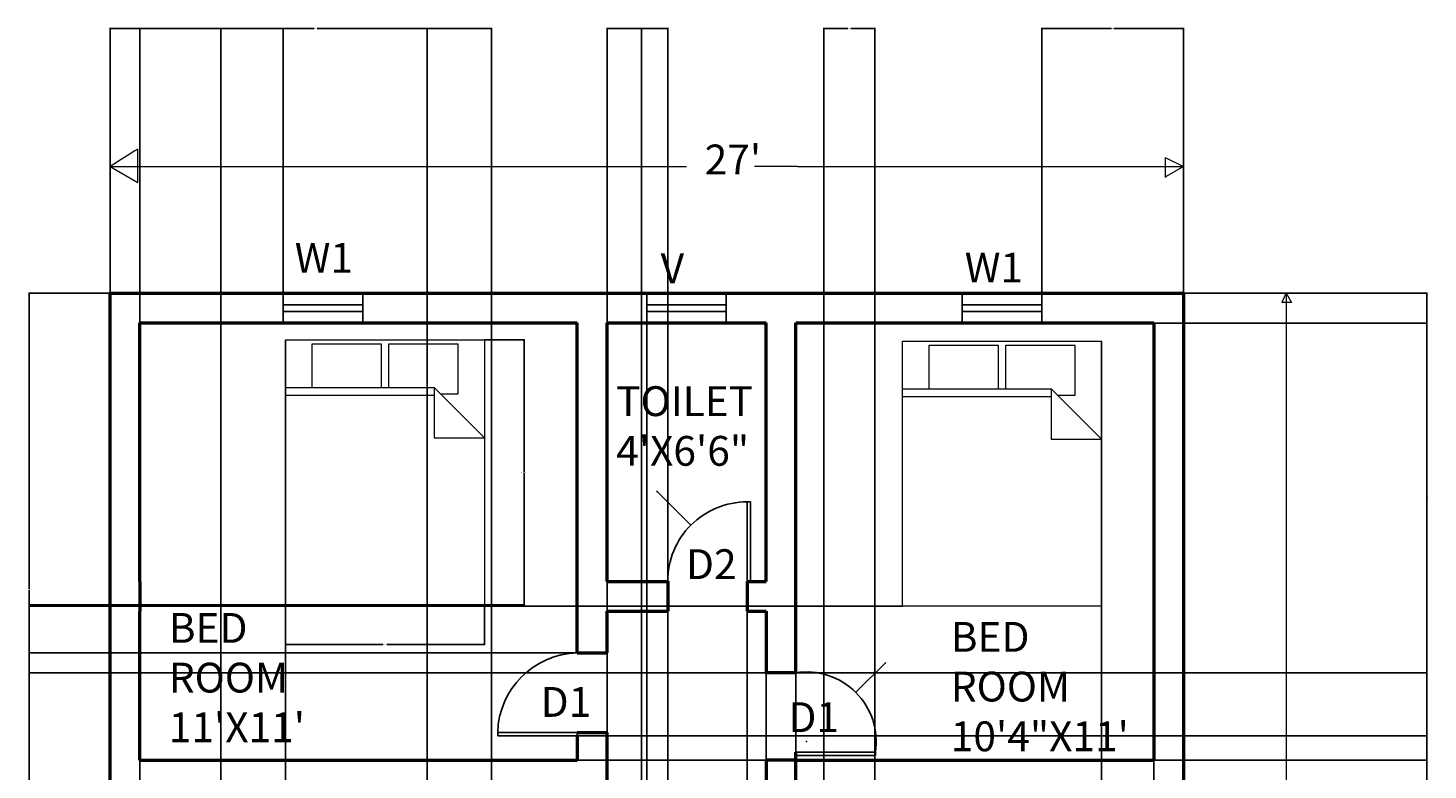
# Model space of a CAD drawing. Units: inches. Extents: x -3 to 419, y -430 to 101.
# Tile 5 of 5: x -3 to 419, y -123 to 101. Entities that reach past the tile are written whole.
import ezdxf

# ---------------------------------------------------------------- set-up
doc = ezdxf.new("R2010")
doc.units = ezdxf.units.IN
doc.header["$MEASUREMENT"] = 0
for name, color, linetype, lineweight in [('A-ANNO-DIMS', 2, 'Continuous', 18), ('A-ANNO-TEXT', 7, 'Continuous', 18), ('A-AREA-IDEN', 7, 'Continuous', 25), ('A-DOOR', 3, 'Continuous', 25), ('A-FURN', 8, 'Continuous', 18), ('A-GLAZ', 4, 'Continuous', 25), ('A-WALL', 7, 'Continuous', 50)]:
    doc.layers.add(name, color=color, linetype=linetype, lineweight=lineweight)
doc.styles.get("Standard").update_dxf_attribs({"font": 'arial.ttf'})
doc.dimstyles.get("Standard").update_dxf_attribs({"dimtxt": 0.18, "dimasz": 0.18, "dimexe": 0.18, "dimexo": 0.0625, "dimgap": 0.09, "dimtad": 0, "dimtih": 1, "dimtoh": 1, "dimdec": 4, "dimzin": 0, "dimdsep": 46, "dimtxsty": 'Standard', "dimcen": 0.09, "dimadec": 0, "dimazin": 0, "dimtfac": 1, "dimtdec": 4, "dimtofl": 0, "dimtmove": 0, "dimatfit": 3, "dimfxl": 1, "dimtolj": 1, "dimtzin": 0, "dimarcsym": 0})

# ---------------------------------------------------------------- blocks, each defined once
blk = doc.blocks.new('Bed - Queen')
for p, q in [((0, -80.00003), (0, 0)), ((0, 0), (59.99999, 0)), ((59.99999, 0), (59.99999, -80.00003)), ((7.99999, -1.2), (28.79998, -1.2)), ((7.99999, -14.4), (7.99999, -1.2)), ((28.79998, -1.2), (28.79998, -14.4)), ((31.19999, -1.2), (51.99999, -1.2)), ((31.19999, -14.4), (31.19999, -1.2)), ((51.99999, -1.2), (51.99999, -16.4)), ((0, -14.4), (44.8, -14.4)), ((44.8, -16.8), (0, -16.8)), ((59.99999, -29.6), (44.8, -14.4)), ((44.8, -14.4), (44.8, -29.6)), ((51.99999, -16.4), (46.79936, -16.4)), ((44.8, -29.6), (59.99999, -29.6)), ((59.99999, -80.00003), (0, -80.00003))]:
    blk.add_line(p, q)
blk = doc.blocks.new('WINDOW-24IN')
for p, q in [((0, 5.5), (24, 5.5)), ((0, 3.5), (24, 3.5))]:
    blk.add_line(p, q)
blk.add_lwpolyline([(0, 9), (24, 9), (24, 0), (0, 0)], close=True)
blk = doc.blocks.new('DOOR-SWING-24IN')
for p, q in [((24, 1), (0, 1)), ((0, 0), (0, 1)), ((24, 0), (0, 0)), ((24, 1), (24, 0))]:
    blk.add_line(p, q)
blk.add_arc((24.7, 0.3), 24.71, 91.6273, 178.3727)
blk = doc.blocks.new('*D11')
at = {"layer": 'A-ANNO-DIMS', "color": 0, "lineweight": -2, "transparency": 16777216}
for p, q in [((134.61, 7.23), (146.72, 7.23)), ((146.54, 7.05), (146.54, -32.58)), ((146.54, -72.59), (146.54, -32.96)), ((134.61, -72.77), (146.72, -72.77))]:
    blk.add_line(p, q, dxfattribs=at)
at = {"layer": 'A-ANNO-DIMS', "color": 0, "transparency": 16777216}
for points in [[(146.51, 7.05), (146.57, 7.05), (146.54, 7.23)], [(146.51, -72.59), (146.57, -72.59), (146.54, -72.77)]]:
    blk.add_solid(points, dxfattribs=at)
at = {"layer": 'Defpoints', "color": 0, "transparency": 16777216}
for p in [(134.54, 7.23), (146.54, 7.23), (134.54, -72.77)]:
    blk.add_point(p, dxfattribs=at)
at = {"layer": 'A-ANNO-DIMS', "color": 0, "transparency": 16777216, "insert": (146.54, -32.77), "char_height": 0.18, "attachment_point": 5}
blk.add_mtext('\\A1;QUEEN BED 80 TYP.', dxfattribs=at)
blk = doc.blocks.new('*D12')
at = {"layer": 'A-ANNO-DIMS', "color": 0, "lineweight": -2, "transparency": 16777216}
for p, q in [((74.54, -72.83), (74.54, -84.95)), ((134.54, -72.83), (134.54, -84.95)), ((74.72, -84.77), (104.02, -84.77)), ((134.36, -84.77), (105.07, -84.77))]:
    blk.add_line(p, q, dxfattribs=at)
at = {"layer": 'A-ANNO-DIMS', "color": 0, "transparency": 16777216}
for points in [[(74.72, -84.74), (74.72, -84.8), (74.54, -84.77)], [(134.36, -84.74), (134.36, -84.8), (134.54, -84.77)]]:
    blk.add_solid(points, dxfattribs=at)
at = {"layer": 'Defpoints', "color": 0, "transparency": 16777216}
for p in [(74.54, -72.77), (134.54, -72.77), (134.54, -84.77)]:
    blk.add_point(p, dxfattribs=at)
at = {"layer": 'A-ANNO-DIMS', "color": 0, "transparency": 16777216, "insert": (104.54, -84.77), "char_height": 0.18, "attachment_point": 5}
blk.add_mtext('\\A1;60 TYP.', dxfattribs=at)
blk = doc.blocks.new('*D25')
at = {"layer": 'A-ANNO-DIMS', "color": 0, "lineweight": -2, "transparency": 16777216}
for p, q in [((21.55, 21.38), (21.55, 101.37)), ((21.73, 101.19), (47.38, 101.19)), ((73.67, 101.19), (48.02, 101.19)), ((73.85, 21.38), (73.85, 101.37))]:
    blk.add_line(p, q, dxfattribs=at)
at = {"layer": 'A-ANNO-DIMS', "color": 0, "transparency": 16777216}
for points in [[(21.73, 101.22), (21.73, 101.16), (21.55, 101.19)], [(73.67, 101.22), (73.67, 101.16), (73.85, 101.19)]]:
    blk.add_solid(points, dxfattribs=at)
at = {"layer": 'Defpoints', "color": 0, "transparency": 16777216}
for p in [(73.85, 101.19), (21.55, 21.31), (73.85, 21.31)]:
    blk.add_point(p, dxfattribs=at)
at = {"layer": 'A-ANNO-DIMS', "color": 0, "transparency": 16777216, "insert": (47.7, 101.19), "char_height": 0.18, "attachment_point": 5}
blk.add_mtext('\\A1;52.3', dxfattribs=at)
blk = doc.blocks.new('*D26')
at = {"layer": 'A-ANNO-DIMS', "color": 0, "lineweight": -2, "transparency": 16777216}
for p, q in [((171.55, 12.25), (171.55, -429.67)), ((183.55, 12.25), (183.55, -429.67)), ((171.73, -429.49), (177.34, -429.49)), ((183.37, -429.49), (177.76, -429.49))]:
    blk.add_line(p, q, dxfattribs=at)
at = {"layer": 'A-ANNO-DIMS', "color": 0, "transparency": 16777216}
for points in [[(171.73, -429.46), (171.73, -429.52), (171.55, -429.49)], [(183.37, -429.46), (183.37, -429.52), (183.55, -429.49)]]:
    blk.add_solid(points, dxfattribs=at)
at = {"layer": 'Defpoints', "color": 0, "transparency": 16777216}
for p in [(171.55, 12.31), (183.55, 12.31), (183.55, -429.49)]:
    blk.add_point(p, dxfattribs=at)
at = {"layer": 'A-ANNO-DIMS', "color": 0, "transparency": 16777216, "insert": (177.55, -429.49), "char_height": 0.18, "attachment_point": 5}
blk.add_mtext('\\A1;12', dxfattribs=at)
blk = doc.blocks.new('*D27')
at = {"layer": 'A-ANNO-DIMS', "color": 0, "lineweight": -2, "transparency": 16777216}
for p, q in [((302.74, 21.38), (302.74, 101.37)), ((302.92, 101.19), (323.77, 101.19)), ((345.37, 101.19), (324.53, 101.19)), ((345.55, 21.38), (345.55, 101.37))]:
    blk.add_line(p, q, dxfattribs=at)
at = {"layer": 'A-ANNO-DIMS', "color": 0, "transparency": 16777216}
for points in [[(302.92, 101.22), (302.92, 101.16), (302.74, 101.19)], [(345.37, 101.22), (345.37, 101.16), (345.55, 101.19)]]:
    blk.add_solid(points, dxfattribs=at)
at = {"layer": 'Defpoints', "color": 0, "transparency": 16777216}
for p in [(345.55, 101.19), (302.74, 21.31), (345.55, 21.31)]:
    blk.add_point(p, dxfattribs=at)
at = {"layer": 'A-ANNO-DIMS', "color": 0, "transparency": 16777216, "insert": (324.15, 101.19), "char_height": 0.18, "attachment_point": 5}
blk.add_mtext('\\A1;42.81', dxfattribs=at)
blk = doc.blocks.new('*D28')
at = {"layer": 'A-ANNO-DIMS', "color": 0, "lineweight": -2, "transparency": 16777216}
for p, q in [((21.49, 21.31), (-3, 21.31)), ((-2.82, 21.13), (-2.82, -67.98)), ((-2.82, -157.46), (-2.82, -68.35)), ((21.49, -157.64), (-3, -157.64))]:
    blk.add_line(p, q, dxfattribs=at)
at = {"layer": 'A-ANNO-DIMS', "color": 0, "transparency": 16777216}
for points in [[(-2.85, 21.13), (-2.79, 21.13), (-2.82, 21.31)], [(-2.85, -157.46), (-2.79, -157.46), (-2.82, -157.64)]]:
    blk.add_solid(points, dxfattribs=at)
at = {"layer": 'Defpoints', "color": 0, "transparency": 16777216}
for p in [(21.55, 21.31), (-2.82, -157.64), (21.55, -157.64)]:
    blk.add_point(p, dxfattribs=at)
at = {"layer": 'A-ANNO-DIMS', "color": 0, "transparency": 16777216, "insert": (-2.82, -68.16), "char_height": 0.18, "attachment_point": 5}
blk.add_mtext('\\A1;178.96', dxfattribs=at)
blk = doc.blocks.new('*D31')
at = {"layer": 'A-ANNO-DIMS', "color": 0, "lineweight": -2, "transparency": 16777216}
for p, q in [((345.62, 21.31), (419.21, 21.31)), ((419.03, 21.13), (419.03, -65.91)), ((419.03, -153.31), (419.03, -66.27)), ((345.62, -153.49), (419.21, -153.49))]:
    blk.add_line(p, q, dxfattribs=at)
at = {"layer": 'A-ANNO-DIMS', "color": 0, "transparency": 16777216}
for points in [[(419, 21.13), (419.06, 21.13), (419.03, 21.31)], [(419, -153.31), (419.06, -153.31), (419.03, -153.49)]]:
    blk.add_solid(points, dxfattribs=at)
at = {"layer": 'Defpoints', "color": 0, "transparency": 16777216}
for p in [(345.55, 21.31), (345.55, -153.49), (419.03, -153.49)]:
    blk.add_point(p, dxfattribs=at)
at = {"layer": 'A-ANNO-DIMS', "color": 0, "transparency": 16777216, "insert": (419.03, -66.09), "char_height": 0.18, "attachment_point": 5}
blk.add_mtext('\\A1;174.8', dxfattribs=at)
blk = doc.blocks.new('*D35')
at = {"layer": 'A-ANNO-DIMS', "color": 0, "lineweight": -2, "transparency": 16777216}
for p, q in [((228.55, 12.25), (228.55, -429.67)), ((336.55, 12.25), (336.55, -429.67)), ((228.73, -429.49), (282.27, -429.49)), ((336.37, -429.49), (282.83, -429.49))]:
    blk.add_line(p, q, dxfattribs=at)
at = {"layer": 'A-ANNO-DIMS', "color": 0, "transparency": 16777216}
for points in [[(228.73, -429.46), (228.73, -429.52), (228.55, -429.49)], [(336.37, -429.46), (336.37, -429.52), (336.55, -429.49)]]:
    blk.add_solid(points, dxfattribs=at)
at = {"layer": 'Defpoints', "color": 0, "transparency": 16777216}
for p in [(228.55, 12.31), (336.55, 12.31), (336.55, -429.49)]:
    blk.add_point(p, dxfattribs=at)
at = {"layer": 'A-ANNO-DIMS', "color": 0, "transparency": 16777216, "insert": (282.55, -429.49), "char_height": 0.18, "attachment_point": 5}
blk.add_mtext('\\A1;108', dxfattribs=at)
blk = doc.blocks.new('*D36')
at = {"layer": 'A-ANNO-DIMS', "color": 0, "lineweight": -2, "transparency": 16777216}
for p, q in [((171.55, -65.62), (171.55, 101.37)), ((171.73, 101.19), (180.25, 101.19)), ((189.68, 101.19), (181.16, 101.19)), ((189.86, -65.62), (189.86, 101.37))]:
    blk.add_line(p, q, dxfattribs=at)
at = {"layer": 'A-ANNO-DIMS', "color": 0, "transparency": 16777216}
for points in [[(171.73, 101.22), (171.73, 101.16), (171.55, 101.19)], [(189.68, 101.22), (189.68, 101.16), (189.86, 101.19)]]:
    blk.add_solid(points, dxfattribs=at)
at = {"layer": 'Defpoints', "color": 0, "transparency": 16777216}
for p in [(189.86, 101.19), (171.55, -65.69), (189.86, -65.69)]:
    blk.add_point(p, dxfattribs=at)
at = {"layer": 'A-ANNO-DIMS', "color": 0, "transparency": 16777216, "insert": (180.71, 101.19), "char_height": 0.18, "attachment_point": 5}
blk.add_mtext('\\A1;18.307', dxfattribs=at)
blk = doc.blocks.new('*D37')
at = {"layer": 'A-ANNO-DIMS', "color": 0, "lineweight": -2, "transparency": 16777216}
for p, q in [((189.86, -65.75), (189.86, -429.67)), ((213.86, -65.75), (213.86, -429.67)), ((190.04, -429.49), (201.64, -429.49)), ((213.68, -429.49), (202.08, -429.49))]:
    blk.add_line(p, q, dxfattribs=at)
at = {"layer": 'A-ANNO-DIMS', "color": 0, "transparency": 16777216}
for points in [[(190.04, -429.46), (190.04, -429.52), (189.86, -429.49)], [(213.68, -429.46), (213.68, -429.52), (213.86, -429.49)]]:
    blk.add_solid(points, dxfattribs=at)
at = {"layer": 'Defpoints', "color": 0, "transparency": 16777216}
for p in [(189.86, -65.69), (213.86, -65.69), (213.86, -429.49)]:
    blk.add_point(p, dxfattribs=at)
at = {"layer": 'A-ANNO-DIMS', "color": 0, "transparency": 16777216, "insert": (201.86, -429.49), "char_height": 0.18, "attachment_point": 5}
blk.add_mtext('\\A1;24', dxfattribs=at)
blk = doc.blocks.new('*D38')
at = {"layer": 'A-ANNO-DIMS', "color": 0, "lineweight": -2, "transparency": 16777216}
for p, q in [((138.62, -112.27), (419.21, -112.27)), ((419.03, -112.45), (419.03, -115.8)), ((419.03, -119.51), (419.03, -116.16)), ((162.62, -119.69), (419.21, -119.69))]:
    blk.add_line(p, q, dxfattribs=at)
at = {"layer": 'A-ANNO-DIMS', "color": 0, "transparency": 16777216}
for points in [[(419, -112.45), (419.06, -112.45), (419.03, -112.27)], [(419, -119.51), (419.06, -119.51), (419.03, -119.69)]]:
    blk.add_solid(points, dxfattribs=at)
at = {"layer": 'Defpoints', "color": 0, "transparency": 16777216}
for p in [(138.55, -112.27), (162.55, -119.69), (419.03, -119.69)]:
    blk.add_point(p, dxfattribs=at)
at = {"layer": 'A-ANNO-DIMS', "color": 0, "transparency": 16777216, "insert": (419.03, -115.98), "char_height": 0.18, "attachment_point": 5}
blk.add_mtext('\\A1;7.416', dxfattribs=at)
blk = doc.blocks.new('*D47')
at = {"layer": 'A-ANNO-DIMS', "color": 0, "lineweight": -2, "transparency": 16777216}
for p, q in [((228.62, 12.31), (419.21, 12.31)), ((419.03, 12.13), (419.03, -40.3)), ((419.03, -93.1), (419.03, -40.66)), ((228.62, -93.28), (419.21, -93.28))]:
    blk.add_line(p, q, dxfattribs=at)
at = {"layer": 'A-ANNO-DIMS', "color": 0, "transparency": 16777216}
for points in [[(419, 12.13), (419.06, 12.13), (419.03, 12.31)], [(419, -93.1), (419.06, -93.1), (419.03, -93.28)]]:
    blk.add_solid(points, dxfattribs=at)
at = {"layer": 'Defpoints', "color": 0, "transparency": 16777216}
for p in [(228.55, 12.31), (228.55, -93.28), (419.03, -93.28)]:
    blk.add_point(p, dxfattribs=at)
at = {"layer": 'A-ANNO-DIMS', "color": 0, "transparency": 16777216, "insert": (419.03, -40.48), "char_height": 0.18, "attachment_point": 5}
blk.add_mtext('\\A1;105.6', dxfattribs=at)
blk = doc.blocks.new('*D48')
at = {"layer": 'A-ANNO-DIMS', "color": 0, "lineweight": -2, "transparency": 16777216}
for p, q in [((30.55, -128.62), (30.55, 101.37)), ((30.73, 101.19), (83.19, 101.19)), ((136.55, 101.19), (84.1, 101.19)), ((136.73, -128.62), (136.73, 101.37))]:
    blk.add_line(p, q, dxfattribs=at)
at = {"layer": 'A-ANNO-DIMS', "color": 0, "transparency": 16777216}
for points in [[(30.73, 101.22), (30.73, 101.16), (30.55, 101.19)], [(136.55, 101.22), (136.55, 101.16), (136.73, 101.19)]]:
    blk.add_solid(points, dxfattribs=at)
at = {"layer": 'Defpoints', "color": 0, "transparency": 16777216}
for p in [(136.73, 101.19), (30.55, -128.69), (136.73, -128.69)]:
    blk.add_point(p, dxfattribs=at)
at = {"layer": 'A-ANNO-DIMS', "color": 0, "transparency": 16777216, "insert": (83.64, 101.19), "char_height": 0.18, "attachment_point": 5}
blk.add_mtext('\\A1;106.18', dxfattribs=at)
blk = doc.blocks.new('*D49')
at = {"layer": 'A-ANNO-DIMS', "color": 0, "lineweight": -2, "transparency": 16777216}
for p, q in [((30.55, -206.62), (30.55, 101.37)), ((30.73, 101.19), (42.38, 101.19)), ((54.82, 101.19), (43.17, 101.19)), ((55, -206.62), (55, 101.37))]:
    blk.add_line(p, q, dxfattribs=at)
at = {"layer": 'A-ANNO-DIMS', "color": 0, "transparency": 16777216}
for points in [[(30.73, 101.22), (30.73, 101.16), (30.55, 101.19)], [(54.82, 101.22), (54.82, 101.16), (55, 101.19)]]:
    blk.add_solid(points, dxfattribs=at)
at = {"layer": 'Defpoints', "color": 0, "transparency": 16777216}
for p in [(55, 101.19), (30.55, -206.69), (55, -206.69)]:
    blk.add_point(p, dxfattribs=at)
at = {"layer": 'A-ANNO-DIMS', "color": 0, "transparency": 16777216, "insert": (42.78, 101.19), "char_height": 0.18, "attachment_point": 5}
blk.add_mtext('\\A1;24.45', dxfattribs=at)
blk = doc.blocks.new('*D52')
at = {"layer": 'A-ANNO-DIMS', "color": 0, "lineweight": -2, "transparency": 16777216}
for p, q in [((117.3, -128.64), (117.3, 101.37)), ((117.48, 101.19), (126.63, 101.19)), ((136.55, 101.19), (127.4, 101.19)), ((136.73, -128.62), (136.73, 101.37))]:
    blk.add_line(p, q, dxfattribs=at)
at = {"layer": 'A-ANNO-DIMS', "color": 0, "transparency": 16777216}
for points in [[(117.48, 101.22), (117.48, 101.16), (117.3, 101.19)], [(136.55, 101.22), (136.55, 101.16), (136.73, 101.19)]]:
    blk.add_solid(points, dxfattribs=at)
at = {"layer": 'Defpoints', "color": 0, "transparency": 16777216}
for p in [(136.73, 101.19), (117.3, -128.7), (136.73, -128.69)]:
    blk.add_point(p, dxfattribs=at)
at = {"layer": 'A-ANNO-DIMS', "color": 0, "transparency": 16777216, "insert": (127.01, 101.19), "char_height": 0.18, "attachment_point": 5}
blk.add_mtext('\\A1;19.43', dxfattribs=at)
blk = doc.blocks.new('*D53')
at = {"layer": 'A-ANNO-DIMS', "color": 0, "lineweight": -2, "transparency": 16777216}
for p, q in [((171.55, -167.61), (171.55, 101.37)), ((171.73, 101.19), (176.3, 101.19)), ((181.78, 101.19), (177.21, 101.19)), ((181.96, -162.84), (181.96, 101.37))]:
    blk.add_line(p, q, dxfattribs=at)
at = {"layer": 'A-ANNO-DIMS', "color": 0, "transparency": 16777216}
for points in [[(171.73, 101.22), (171.73, 101.16), (171.55, 101.19)], [(181.78, 101.22), (181.78, 101.16), (181.96, 101.19)]]:
    blk.add_solid(points, dxfattribs=at)
at = {"layer": 'Defpoints', "color": 0, "transparency": 16777216}
for p in [(181.96, 101.19), (181.96, -162.9), (171.55, -167.67)]:
    blk.add_point(p, dxfattribs=at)
at = {"layer": 'A-ANNO-DIMS', "color": 0, "transparency": 16777216, "insert": (176.76, 101.19), "char_height": 0.18, "attachment_point": 5}
blk.add_mtext('\\A1;10.407', dxfattribs=at)
blk = doc.blocks.new('*D56')
at = {"layer": 'A-ANNO-DIMS', "color": 0, "lineweight": -2, "transparency": 16777216}
for p, q in [((236.96, -162.84), (236.96, 101.37)), ((237.14, 101.19), (244.22, 101.19)), ((252.22, 101.19), (245.13, 101.19)), ((252.4, -155.79), (252.4, 101.37))]:
    blk.add_line(p, q, dxfattribs=at)
at = {"layer": 'A-ANNO-DIMS', "color": 0, "transparency": 16777216}
for points in [[(237.14, 101.22), (237.14, 101.16), (236.96, 101.19)], [(252.22, 101.22), (252.22, 101.16), (252.4, 101.19)]]:
    blk.add_solid(points, dxfattribs=at)
at = {"layer": 'Defpoints', "color": 0, "transparency": 16777216}
for p in [(236.96, 101.19), (252.4, -155.85), (236.96, -162.9)]:
    blk.add_point(p, dxfattribs=at)
at = {"layer": 'A-ANNO-DIMS', "color": 0, "transparency": 16777216, "insert": (244.68, 101.19), "char_height": 0.18, "attachment_point": 5}
blk.add_mtext('\\A1;15.438', dxfattribs=at)
blk = doc.blocks.new('*D59')
at = {"layer": 'A-ANNO-DIMS', "color": 0, "lineweight": -2, "transparency": 16777216}
for p, q in [((30.55, 12.25), (30.55, -429.67)), ((74.54, 7.17), (74.54, -429.67)), ((30.73, -429.49), (52.15, -429.49)), ((74.36, -429.49), (52.95, -429.49))]:
    blk.add_line(p, q, dxfattribs=at)
at = {"layer": 'A-ANNO-DIMS', "color": 0, "transparency": 16777216}
for points in [[(30.73, -429.46), (30.73, -429.52), (30.55, -429.49)], [(74.36, -429.46), (74.36, -429.52), (74.54, -429.49)]]:
    blk.add_solid(points, dxfattribs=at)
at = {"layer": 'Defpoints', "color": 0, "transparency": 16777216}
for p in [(30.55, 12.31), (74.54, 7.23), (74.54, -429.49)]:
    blk.add_point(p, dxfattribs=at)
at = {"layer": 'A-ANNO-DIMS', "color": 0, "transparency": 16777216, "insert": (52.55, -429.49), "char_height": 0.18, "attachment_point": 5}
blk.add_mtext('\\A1;43.99', dxfattribs=at)
blk = doc.blocks.new('*D61')
at = {"layer": 'A-ANNO-DIMS', "color": 0, "lineweight": -2, "transparency": 16777216}
for p, q in [((336.55, 12.25), (336.55, -429.67)), ((320.77, 6.77), (320.77, -429.67)), ((320.95, -429.49), (328.21, -429.49)), ((336.37, -429.49), (329.12, -429.49))]:
    blk.add_line(p, q, dxfattribs=at)
at = {"layer": 'A-ANNO-DIMS', "color": 0, "transparency": 16777216}
for points in [[(320.95, -429.46), (320.95, -429.52), (320.77, -429.49)], [(336.37, -429.46), (336.37, -429.52), (336.55, -429.49)]]:
    blk.add_solid(points, dxfattribs=at)
at = {"layer": 'Defpoints', "color": 0, "transparency": 16777216}
for p in [(336.55, 12.31), (320.77, 6.83), (320.77, -429.49)]:
    blk.add_point(p, dxfattribs=at)
at = {"layer": 'A-ANNO-DIMS', "color": 0, "transparency": 16777216, "insert": (328.66, -429.49), "char_height": 0.18, "attachment_point": 5}
blk.add_mtext('\\A1;15.783', dxfattribs=at)
blk = doc.blocks.new('*D62')
at = {"layer": 'A-ANNO-DIMS', "color": 0, "lineweight": -2, "transparency": 16777216}
for p, q in [((134.48, -72.77), (-3, -72.77)), ((-2.82, -72.95), (-2.82, -79.84)), ((-2.82, -87.09), (-2.82, -80.2)), ((162.49, -87.27), (-3, -87.27))]:
    blk.add_line(p, q, dxfattribs=at)
at = {"layer": 'A-ANNO-DIMS', "color": 0, "transparency": 16777216}
for points in [[(-2.85, -72.95), (-2.79, -72.95), (-2.82, -72.77)], [(-2.85, -87.09), (-2.79, -87.09), (-2.82, -87.27)]]:
    blk.add_solid(points, dxfattribs=at)
at = {"layer": 'Defpoints', "color": 0, "transparency": 16777216}
for p in [(134.54, -72.77), (-2.82, -87.27), (162.55, -87.27)]:
    blk.add_point(p, dxfattribs=at)
at = {"layer": 'A-ANNO-DIMS', "color": 0, "transparency": 16777216, "insert": (-2.82, -80.02), "char_height": 0.18, "attachment_point": 5}
blk.add_mtext('\\A1;14.5', dxfattribs=at)
blk = doc.blocks.new('*D63')
at = {"layer": 'A-ANNO-DIMS', "color": 0, "lineweight": -2, "transparency": 16777216}
for p, q in [((260.71, -73.17), (-3, -73.17)), ((-2.82, -73.35), (-2.82, -83.04)), ((-2.82, -93.1), (-2.82, -83.4)), ((228.49, -93.28), (-3, -93.28))]:
    blk.add_line(p, q, dxfattribs=at)
at = {"layer": 'A-ANNO-DIMS', "color": 0, "transparency": 16777216}
for points in [[(-2.85, -73.35), (-2.79, -73.35), (-2.82, -73.17)], [(-2.85, -93.1), (-2.79, -93.1), (-2.82, -93.28)]]:
    blk.add_solid(points, dxfattribs=at)
at = {"layer": 'Defpoints', "color": 0, "transparency": 16777216}
for p in [(260.77, -73.17), (-2.82, -93.28), (228.55, -93.28)]:
    blk.add_point(p, dxfattribs=at)
at = {"layer": 'A-ANNO-DIMS', "color": 0, "transparency": 16777216, "insert": (-2.82, -83.22), "char_height": 0.18, "attachment_point": 5}
blk.add_mtext('\\A1;20.11', dxfattribs=at)
blk = doc.blocks.new('*D71')
at = {"layer": 'A-ANNO-DIMS', "color": 0, "lineweight": -2, "transparency": 16777216}
for p, q in [((186.53, -38.54), (186.71, -38.54)), ((186.71, -38.54), (196.75, -48.58)), ((213.73, -65.65), (213.91, -65.65)), ((213.82, -65.74), (213.82, -65.56))]:
    blk.add_line(p, q, dxfattribs=at)
at = {"layer": 'A-ANNO-DIMS', "color": 0, "transparency": 16777216}
blk.add_solid([(196.77, -48.55), (196.73, -48.6), (196.88, -48.7)], dxfattribs=at)
at = {"layer": 'Defpoints', "color": 0, "transparency": 16777216}
for p in [(196.88, -48.7), (213.82, -65.65)]:
    blk.add_point(p, dxfattribs=at)
at = {"layer": 'A-ANNO-DIMS', "color": 0, "transparency": 16777216, "insert": (186.05, -38.54), "char_height": 0.18, "attachment_point": 5}
blk.add_mtext('\\A1;R23.96', dxfattribs=at)
blk = doc.blocks.new('*D73')
at = {"layer": 'A-ANNO-DIMS', "color": 0, "lineweight": -2, "transparency": 16777216}
for p, q in [((255.56, -90.27), (246.77, -99.06)), ((255.74, -90.27), (255.56, -90.27)), ((231.68, -114.06), (231.86, -114.06)), ((231.77, -114.15), (231.77, -113.97))]:
    blk.add_line(p, q, dxfattribs=at)
at = {"layer": 'A-ANNO-DIMS', "color": 0, "transparency": 16777216}
blk.add_solid([(246.75, -99.04), (246.79, -99.08), (246.64, -99.19)], dxfattribs=at)
at = {"layer": 'Defpoints', "color": 0, "transparency": 16777216}
for p in [(246.64, -99.19), (231.77, -114.06)]:
    blk.add_point(p, dxfattribs=at)
at = {"layer": 'A-ANNO-DIMS', "color": 0, "transparency": 16777216, "insert": (256.22, -90.27), "char_height": 0.18, "attachment_point": 5}
blk.add_mtext('\\A1;R21.03', dxfattribs=at)

msp = doc.modelspace()

# ---------------------------------------------------------------- linework, layer by layer
at = {"layer": 'A-ANNO-DIMS'}
for p, q in [((21.5532, 42.9459), (21.5532, 76.2488)), ((345.5532, 59.5974), (345.5532, 76.8133)), ((29.065, 64.3085), (21.5532, 59.5974)), ((29.9087, 64.8377), (29.065, 64.3085)), ((29.9087, 54.7733), (29.9087, 64.8377)), ((21.5532, 59.5974), (179.3407, 59.5974)), ((21.5532, 59.5974), (29.9087, 54.7733)), ((179.3407, 59.5974), (195.542, 59.5974)), ((229.071, 59.5974), (216.0787, 59.5974)), ((229.071, 59.5974), (345.5532, 59.5974)), ((339.9772, 62.3068), (345.5532, 59.5974)), ((339.9772, 62.3068), (339.9772, 56.3781)), ((345.5532, 59.5974), (340.2891, 56.5582)), ((345.5532, 59.5974), (345.5532, 42.3815)), ((339.9772, 56.3781), (340.2891, 56.5582)), ((358.4827, 21.3147), (394.6501, 21.3147)), ((375.2731, 18.5665), (376.5664, 21.3147)), ((376.5664, 21.3147), (378.1768, 18.5255)), ((376.5664, 21.3147), (376.5664, -183.7646)), ((375.2384, 18.5255), (375.2731, 18.5665)), ((375.3602, 18.5255), (375.2384, 18.5255)), ((375.2731, 18.5665), (375.2731, 18.5665)), ((378.1768, 18.5255), (375.3602, 18.5255))]:
    msp.add_line(p, q, dxfattribs=at)
at = {"layer": 'A-DOOR'}
for p, q in [((213.8603, -65.6853), (213.8603, -41.6853)), ((213.8603, -41.6853), (214.8603, -41.6853)), ((214.8603, -65.6853), (214.8603, -41.6853)), ((213.8603, -65.6853), (214.8603, -65.6853)), ((171.5532, -111.2695), (171.5532, -87.2695)), ((219.5532, -93.277), (219.5532, -119.6853)), ((228.5532, -117.277), (252.5532, -117.277)), ((228.5532, -117.277), (228.5532, -118.277)), ((228.5532, -118.277), (252.5532, -118.277)), ((252.5532, -117.277), (252.5532, -118.277))]:
    msp.add_line(p, q, dxfattribs=at)
for centre, radius, start, end in [((213.8211, -65.6461), 23.9608, 89.906283, 180.093717), ((231.7703, -114.0598), 21.0304, 351.200553, 98.799447)]:
    msp.add_arc(centre, radius, start, end, dxfattribs=at)
at = {"layer": 'A-WALL'}
for p, q in [((30.5532, 12.3147), (162.5532, 12.3147)), ((30.5532, -65.6853), (30.5532, 12.3147)), ((162.5532, -87.2695), (162.5532, 12.3147)), ((171.5532, 12.3147), (219.5532, 12.3147)), ((171.5532, -65.6853), (171.5532, 12.3147)), ((219.5532, -65.6853), (219.5532, 12.3147)), ((219.5532, -65.6853), (219.5532, 12.3147)), ((228.5532, -74.6853), (228.5532, 12.3147)), ((228.5532, 12.3147), (336.5532, 12.3147)), ((228.5532, -93.277), (228.5532, 12.3147)), ((336.5532, 12.3147), (336.5532, -65.6853)), ((30.5532, -65.6853), (30.5532, -74.6853)), ((171.5532, -65.6853), (189.8603, -65.6853)), ((189.8603, -65.6461), (189.8603, -74.6853)), ((213.8603, -65.6853), (213.8603, -74.6853)), ((213.8603, -65.6853), (219.5532, -65.6853)), ((336.5532, -65.6853), (336.5532, -74.6853)), ((30.5532, -119.6853), (30.5532, -74.6853)), ((171.5532, -74.6853), (189.8603, -74.6853)), ((171.5532, -87.2695), (171.5532, -74.6853)), ((213.8603, -74.6853), (219.5532, -74.6853)), ((219.5532, -74.6853), (219.5532, -93.277)), ((336.5532, -74.6853), (336.5532, -119.6853)), ((162.5532, -87.2695), (171.5532, -87.2695)), ((228.5532, -93.277), (219.5532, -93.277)), ((162.5532, -111.2695), (171.5532, -111.2695)), ((162.5532, -112.2695), (162.5532, -119.6853)), ((171.5532, -167.6713), (171.5532, -111.2695)), ((228.5532, -128.6853), (228.5532, -117.277)), ((30.5532, -119.6853), (162.5532, -119.6853)), ((228.5532, -119.6853), (219.5532, -119.6853)), ((219.5532, -119.6853), (219.5532, -128.6853)), ((228.5532, -119.6853), (336.5532, -119.6853))]:
    msp.add_line(p, q, dxfattribs=at)
msp.add_lwpolyline([(266.5221, -404.6853), (21.5532, -404.6853), (21.5532, 21.3147), (345.5532, 21.3147), (345.5532, -404.6853)], dxfattribs=at)

# ---------------------------------------------------------------- block references
at = {"layer": 'A-DOOR'}
msp.add_blockref('DOOR-SWING-24IN', (138.553, -112.27), dxfattribs=at)
at = {"layer": 'A-FURN'}
for p in [(74.5439, 7.23), (260.7704, 6.8316)]:
    msp.add_blockref('Bed - Queen', p, dxfattribs=at)
at = {"layer": 'A-GLAZ'}
for p in [(73.849, 12.315), (183.5533, 12.315), (278.7441, 12.315)]:
    msp.add_blockref('WINDOW-24IN', p, dxfattribs=at)

# ---------------------------------------------------------------- texts
at = {"layer": 'A-ANNO-DIMS', "insert": (201.0343, 66.1741), "char_height": 9, "attachment_point": 1}
msp.add_mtext_dynamic_manual_height_columns("27'", width=35.194991, gutter_width=45, heights=[0], dxfattribs=at)
at = {"layer": 'A-ANNO-TEXT', "char_height": 9, "attachment_point": 1}
for s, width, insert in [('W1', 27.895294, (77.2977, 36.4872)), ('V', 33.840188, (187.7445, 33.3204)), ('W1', 29.724494, (279.5236, 33.5597)), ('D2', 5.399497, (195.4027, -55.9885)), ('D1', 14.100742, (151.5284, -97.5768)), ('D1', 20.237951, (226.3079, -102.1868))]:
    msp.add_mtext_dynamic_manual_height_columns(s, width=width, gutter_width=45, heights=[0], dxfattribs=dict(at, insert=insert))
at = {"layer": 'A-AREA-IDEN', "char_height": 9, "attachment_point": 1}
for s, width, insert in [('TOILET\\P4\'X6\'6"', 25.501317, (174.3216, -6.7784)), ("BED ROOM\\P11'X11'", 62.37827, (39.298, -75.2341)), ('BED ROOM\\P10\'4"X11\'', 53.195013, (275.3115, -77.9478))]:
    msp.add_mtext_dynamic_manual_height_columns(s, width=width, gutter_width=45, heights=[0], dxfattribs=dict(at, insert=insert))

# ---------------------------------------------------------------- dimensions: what is measured, and where the dimension line sits
at = {"layer": 'A-ANNO-DIMS'}
for base, p1, p2, override, picture, middle in [((73.8488, 101.1903), (21.5532, 21.3147), (73.8488, 21.3147), {"dimdec": 1, "dimlfac": 1, "dimrnd": 0, "dimzin": 0, "dimdsep": 46, "dimlunit": 2}, '*D25', (47.701, 101.1903)), ((136.73, 101.1903), (30.5532, -128.6853), (136.73, -128.6853), {"dimdec": 2, "dimlfac": 1, "dimrnd": 0, "dimzin": 0, "dimdsep": 46, "dimlunit": 2}, '*D48', (83.6416, 101.1903)), ((55.004, 101.1903), (30.5532, -206.6853), (55.004, -206.6853), {"dimdec": 2, "dimlfac": 1, "dimrnd": 0, "dimzin": 0, "dimdsep": 46, "dimlunit": 2}, '*D49', (42.7786, 101.1903)), ((136.73, 101.1903), (117.2993, -128.7009), (136.73, -128.6853), {"dimdec": 2, "dimlfac": 1, "dimrnd": 0, "dimzin": 0, "dimdsep": 46, "dimlunit": 2}, '*D52', (127.0147, 101.1903)), ((189.8603, 101.1903), (171.5532, -65.6853), (189.8603, -65.6853), {"dimdec": 3, "dimlfac": 1, "dimrnd": 0, "dimzin": 0, "dimdsep": 46, "dimlunit": 2}, '*D36', (180.7067, 101.1903)), ((181.9598, 101.1903), (171.5532, -167.6713), (181.9598, -162.8988), {"dimdec": 3, "dimlfac": 1, "dimrnd": 0, "dimzin": 0, "dimdsep": 46, "dimlunit": 2}, '*D53', (176.7565, 101.1903)), ((236.9598, 101.1903), (252.3974, -155.8529), (236.9598, -162.8988), {"dimdec": 3, "dimlfac": 1, "dimrnd": 0, "dimzin": 0, "dimdsep": 46, "dimlunit": 2}, '*D56', (244.6786, 101.1903)), ((345.5532, 101.1903), (302.744, 21.3147), (345.5532, 21.3147), {"dimdec": 2, "dimlfac": 1, "dimrnd": 0, "dimzin": 0, "dimdsep": 46, "dimlunit": 2}, '*D27', (324.1486, 101.1903)), ((74.5439, -429.4854), (30.5532, 12.3147), (74.5439, 7.23), {"dimdec": 2, "dimlfac": 1, "dimrnd": 0, "dimzin": 0, "dimdsep": 46, "dimlunit": 2}, '*D59', (52.5485, -429.4854)), ((183.5532, -429.4854), (171.5532, 12.3147), (183.5532, 12.3147), {"dimdec": 0, "dimlfac": 1, "dimrnd": 0, "dimzin": 0, "dimdsep": 46, "dimlunit": 2}, '*D26', (177.5532, -429.4854)), ((336.5532, -429.4854), (228.5532, 12.3147), (336.5532, 12.3147), {"dimdec": 0, "dimlfac": 1, "dimrnd": 0, "dimzin": 0, "dimdsep": 46, "dimlunit": 2}, '*D35', (282.5532, -429.4854)), ((320.7704, -429.4854), (336.5532, 12.3147), (320.7704, 6.8316), {"dimdec": 3, "dimlfac": 1, "dimrnd": 0, "dimzin": 0, "dimdsep": 46, "dimlunit": 2}, '*D61', (328.6618, -429.4854)), ((213.8603, -429.4854), (189.8603, -65.6853), (213.8603, -65.6853), {"dimdec": 0, "dimlfac": 1, "dimrnd": 0, "dimzin": 0, "dimdsep": 46, "dimlunit": 2}, '*D37', (201.8603, -429.4854))]:
    dim = msp.add_linear_dim(base=base, p1=p1, p2=p2, dimstyle='Standard', override=override, dxfattribs=at)
    dim.commit()
    dim.dimension.update_dxf_attribs({"geometry": picture, "text_midpoint": middle})
for base, p1, p2, override, picture, middle in [((-2.8238, -157.6432), (21.5532, 21.3147), (21.5532, -157.6432), {"dimdec": 2, "dimlfac": 1, "dimrnd": 0, "dimzin": 0, "dimdsep": 46, "dimlunit": 2}, '*D28', (-2.8238, -68.1642)), ((419.0271, -153.4893), (345.5532, 21.3147), (345.5532, -153.4893), {"dimdec": 1, "dimlfac": 1, "dimrnd": 0, "dimzin": 0, "dimdsep": 46, "dimlunit": 2}, '*D31', (419.0271, -66.0873)), ((419.0271, -93.277), (228.5532, 12.3147), (228.5532, -93.277), {"dimdec": 1, "dimlfac": 1, "dimrnd": 0, "dimzin": 0, "dimdsep": 46, "dimlunit": 2}, '*D47', (419.0271, -40.4811)), ((-2.8238, -93.277), (260.7704, -73.1684), (228.5532, -93.277), {"dimdec": 2, "dimlfac": 1, "dimrnd": 0, "dimzin": 0, "dimdsep": 46, "dimlunit": 2}, '*D63', (-2.8238, -83.2227)), ((-2.8238, -87.2695), (134.5439, -72.77), (162.5532, -87.2695), {"dimdec": 1, "dimlfac": 1, "dimrnd": 0, "dimzin": 0, "dimdsep": 46, "dimlunit": 2}, '*D62', (-2.8238, -80.0198)), ((419.0271, -119.6853), (138.5532, -112.2695), (162.5532, -119.6853), {"dimdec": 3, "dimlfac": 1, "dimrnd": 0, "dimzin": 0, "dimdsep": 46, "dimlunit": 2}, '*D38', (419.0271, -115.9774))]:
    dim = msp.add_linear_dim(base=base, p1=p1, p2=p2, angle=90, dimstyle='Standard', override=override, dxfattribs=at)
    dim.commit()
    dim.dimension.update_dxf_attribs({"geometry": picture, "text_midpoint": middle})
dim = msp.add_linear_dim(base=(146.5439, 7.23), p1=(134.5439, -72.77), p2=(134.5439, 7.23), angle=90, text='QUEEN BED <> TYP.', dimstyle='Standard', override={"dimdec": 0, "dimlfac": 1, "dimrnd": 0, "dimzin": 0, "dimdsep": 46, "dimlunit": 2}, dxfattribs=at)
dim.commit()
dim.dimension.update_dxf_attribs({"geometry": '*D11', "text_midpoint": (146.5439, -32.77)})
for center, mpoint, picture, middle in [((213.8211, -65.6461), (196.8782, -48.7032), '*D71', (186.0527, -38.5375)), ((231.7703, -114.0598), (246.641, -99.189), '*D73', (256.2232, -90.2665))]:
    dim = msp.add_radius_dim(center=center, mpoint=mpoint, dimstyle='Standard', override={"dimdec": 2, "dimlfac": 1, "dimrnd": 0, "dimzin": 0, "dimdsep": 46, "dimlunit": 2}, dxfattribs=at)
    dim.commit()
    dim.dimension.update_dxf_attribs({"geometry": picture, "text_midpoint": middle, "dimtype": 164})
dim = msp.add_linear_dim(base=(134.5439, -84.77), p1=(74.5439, -72.77), p2=(134.5439, -72.77), text='<> TYP.', dimstyle='Standard', override={"dimdec": 0, "dimlfac": 1, "dimrnd": 0, "dimzin": 0, "dimdsep": 46, "dimlunit": 2}, dxfattribs=at)
dim.commit()
dim.dimension.update_dxf_attribs({"geometry": '*D12', "text_midpoint": (104.5439, -84.77)})

doc.saveas('drawing.dxf')
